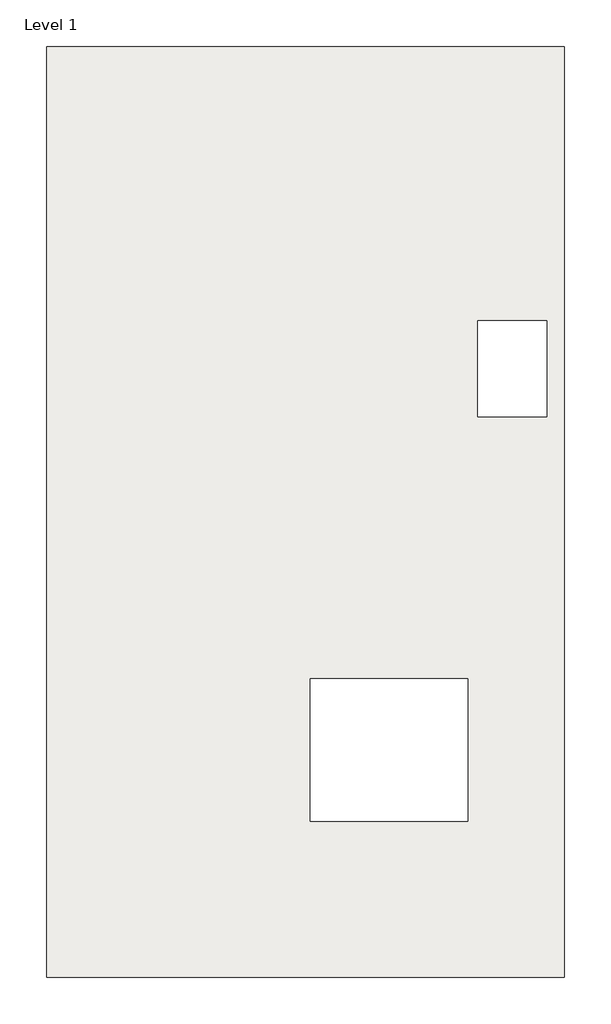
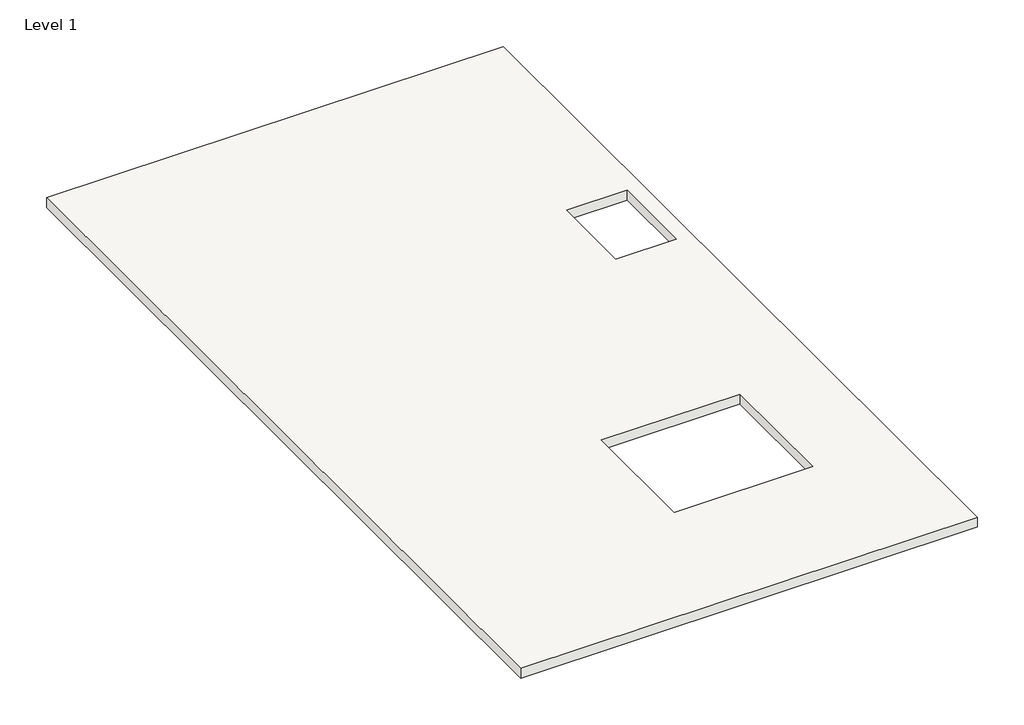
# One storey: 1 slab.
"""IFC4 building model written with IfcOpenShell, lengths in millimetres."""

from ifc_helpers import new_model, si_unit, frame, origin, place, context, project, spatial, polyline, outline, extrude, element, save

model = new_model("IFC4")

# Units and contexts
model_context = context("Model", 3, world=origin())
ifc_project = project(units=[si_unit("LENGTHUNIT", "METRE", prefix="MILLI")], contexts=[model_context])

# Site, building, storey
site = spatial("IfcSite", under=ifc_project)
building = spatial("IfcBuilding", under=site)
storey = spatial("IfcBuildingStorey", under=building, Name="Level 1", Elevation=4000.0)

# Slab
placement = place(None, origin())
element("IfcSlab", 1, ObjectType="Standard", at=placement, inside=storey, context=model_context, shape_type="SweptSolid", body=[
    extrude(outline(polyline([(6011.1511137, 11833.2891038), (6011.1511137, -12132.0352742), (-7317.4988863, -12132.0352742), (-7317.4988863, 11833.2891038), (6011.1511137, 11833.2891038)]), holes=[polyline([(3521.6011137, -4436.6352742), (-522.9988863, -4436.6352742), (-522.9988863, -8115.821978), (3521.6011137, -8115.821978), (3521.6011137, -4436.6352742)]), polyline([(5553.9511137, 4777.5566744), (3788.6511137, 4777.5566744), (3788.6511137, 2296.7809218), (5553.9511137, 2296.7809218), (5553.9511137, 4777.5566744)])]), frame((0.0, 0.0, 3700.0), z_axis=(0.0, 0.0, 1.0), x_axis=(1.0, 0.0, 0.0)), (0.0, 0.0, 1.0), 300.0),
])

save(model, "model.ifc")

# Revit data of these elements
# Type "Standard"
#   Layers, outside or top first: 300 mm no material (function 1)
# Element 1 (IfcSlab, "Standard")
#   Height Offset From Level = 0 mm
#   built-in parameter 1001954 = 1
#   Phase Created = New Construction
